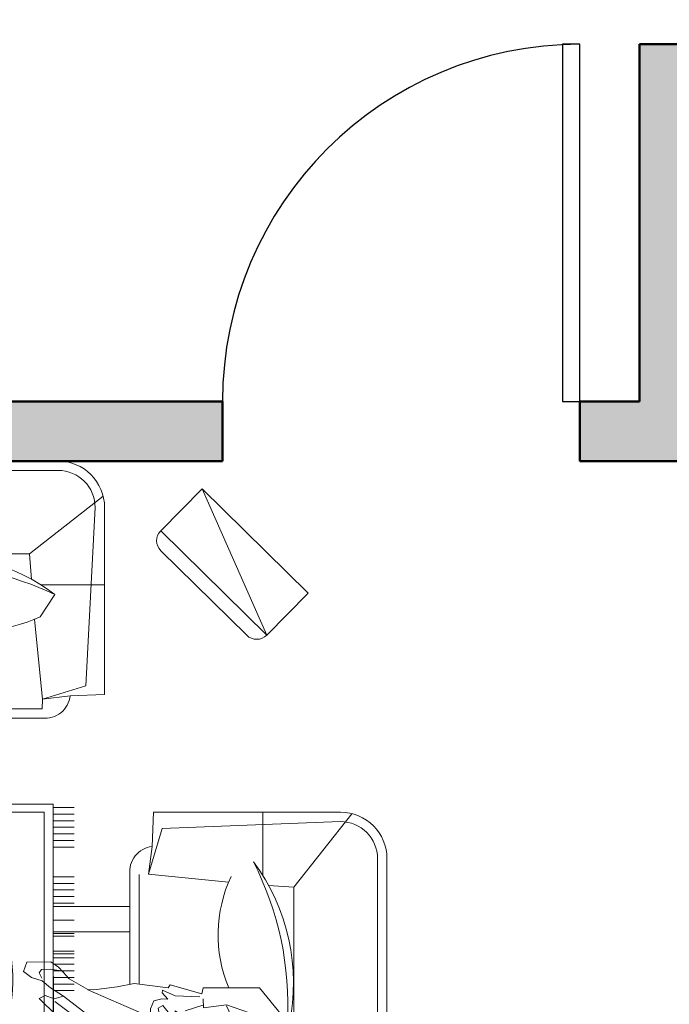
# Model space of a CAD drawing. Units: inches. Extents: x 375 to 1122, y 27 to 1069.
# Tile 70 of 155: x 601 to 667, y 400 to 499. Entities that reach past the tile are written whole.
import ezdxf

# ---------------------------------------------------------------- set-up
doc = ezdxf.new("R2010")
doc.units = ezdxf.units.IN
for name, color, linetype, lineweight in [('A-ANNO-DIMS', 2, 'Continuous', 18), ('A-WALL-PATT', 252, 'Continuous', 13), ('Doors', 150, 'Continuous', 25), ('Furniture', 30, 'Continuous', 18), ('Walls', 250, 'Continuous', 50)]:
    doc.layers.add(name, color=color, linetype=linetype, lineweight=lineweight)
doc.styles.get("Standard").update_dxf_attribs({"font": 'arial.ttf'})
doc.dimstyles.new('ISO-25', dxfattribs={"dimtxt": 12, "dimasz": 2.5, "dimexe": 1.5, "dimexo": 1.5, "dimtad": 1, "dimdec": 1, "dimlunit": 3, "dimtxsty": 'Standard', "dimblk": 'ARCHTICK', "dimcen": 2.5, "dimadec": 0, "dimazin": 0, "dimtfac": 1, "dimtdec": 1, "dimtmove": 0, "dimatfit": 3, "dimfxl": 1.5, "dimfxlon": 1, "dimarcsym": 0})

# ---------------------------------------------------------------- blocks, each defined once
blk = doc.blocks.new('*U9')
for p, q in [((-36, 0), (-36, -4)), ((0, 0), (0, -4))]:
    blk.add_line(p, q)
blk.add_lwpolyline([(0, 0), (0, 36), (-1.75, 36), (-1.75, 0)], close=True)
blk.add_arc((0, 0), 36, 90, 180)
blk = doc.blocks.new('*U11')
for p, q in [((-24, 0), (-24, -4)), ((0, 0), (0, -4))]:
    blk.add_line(p, q)
blk.add_lwpolyline([(0, 0), (0, 24), (-1.75, 24), (-1.75, 0)], close=True)
blk.add_arc((0, 0), 24, 90, 180)
blk = doc.blocks.new('A$C4DC51D13')
for p, q in [((3265.3, 2996.2), (1188.4, 2996.2)), ((1895.2, 2134), (1895.2, 2996.2)), ((2559.6, 2996.2), (2559.6, 2617.8)), ((1188.4, 2962.7), (1862.1, 2962.7)), ((1862.1, 2134), (1862.1, 2962.7)), ((1928.3, 2961.6), (2524.2, 2961.6)), ((1928.3, 2134), (1928.3, 2961.6)), ((2524.2, 2961.6), (2524.2, 2658.6)), ((2590.4, 2962.7), (2590.4, 2654.5)), ((3265.3, 2962.7), (2590.4, 2962.7)), ((277.4, 2939.6), (277.4, 2141.8)), ((943, 2103.5), (943, 2936.7)), ((1018.2, 2892.3), (232.2, 2892.3)), ((3778.5, 2897), (3631.2, 2747.3)), ((4008.9, 2375.5), (3778.5, 2897)), ((4156.2, 2525.2), (3778.5, 2897)), ((304, 2865.7), (304, 2253.3)), ((916.4, 2865.7), (304, 2865.7)), ((916.4, 2253.3), (916.4, 2865.7)), ((1290.4, 2664.8), (1028, 2870.9)), ((3163.3, 2664.8), (3425.7, 2870.9)), ((1022.9, 2163.8), (1022.9, 2830.3)), ((1056, 2830.3), (1081, 2194.8)), ((3397.7, 2830.3), (3364.5, 2194.8)), ((3430.8, 2163.8), (3430.8, 2830.3)), ((4008.9, 2375.5), (3631.2, 2747.3)), ((423.7, 2370.8), (776.6, 2723.7)), ((427.4, 2727.4), (772.8, 2367.1)), ((506.4, 2652.2), (506.4, 2704.4)), ((510.6, 2655.8), (510.6, 2706.9)), ((514.9, 2659.2), (514.9, 2709.2)), ((519.1, 2662.3), (519.1, 2711.3)), ((523.3, 2665.1), (523.3, 2713.4)), ((527.5, 2667.8), (527.5, 2715.2)), ((531.8, 2670.2), (531.8, 2717)), ((536, 2672.5), (536, 2718.7)), ((540.2, 2674.6), (540.2, 2720.2)), ((544.4, 2676.5), (544.4, 2721.6)), ((548.7, 2678.2), (548.7, 2722.9)), ((650.1, 2678.8), (650.1, 2723.3)), ((654.3, 2677.1), (654.3, 2722)), ((658.6, 2675.2), (658.6, 2720.7)), ((662.8, 2673.2), (662.8, 2719.2)), ((667, 2671), (667, 2717.6)), ((668.5, 2670.2), (668.5, 2717)), ((671.2, 2668.6), (671.2, 2715.9)), ((672.7, 2667.8), (672.7, 2715.2)), ((675.5, 2666.1), (675.5, 2714)), ((676.9, 2665.1), (676.9, 2713.4)), ((679.7, 2663.3), (679.7, 2712)), ((681.1, 2662.3), (681.1, 2711.3)), ((683.9, 2660.3), (683.9, 2709.9)), ((685.4, 2659.2), (685.4, 2709.2)), ((688.1, 2657), (688.1, 2707.7)), ((689.6, 2655.8), (689.6, 2706.9)), ((692.4, 2653.5), (692.4, 2705.3)), ((693.8, 2652.2), (693.8, 2704.4)), ((464.1, 2583.3), (464.1, 2669.7)), ((465.8, 2671.5), (534.1, 2671.5)), ((468.4, 2596.6), (468.4, 2674.3)), ((469.8, 2675.7), (542.8, 2675.7)), ((472.6, 2606.7), (472.6, 2678.5)), ((476.8, 2615), (476.8, 2682.5)), ((481, 2622.2), (481, 2686.2)), ((485.3, 2628.5), (485.3, 2689.7)), ((489.5, 2634.2), (489.5, 2693)), ((493.7, 2639.3), (493.7, 2696.1)), ((497.9, 2644), (497.9, 2699.1)), ((502.2, 2648.3), (502.2, 2701.8)), ((657.4, 2675.7), (730.4, 2675.7)), ((734.5, 2671.5), (666.1, 2671.5)), ((666.1, 2671.5), (734.5, 2671.5)), ((696.6, 2649.6), (696.6, 2702.7)), ((698, 2648.3), (698, 2701.8)), ((700.8, 2645.5), (700.8, 2700)), ((702.3, 2644), (702.3, 2699.1)), ((705, 2641), (705, 2697.2)), ((706.5, 2639.3), (706.5, 2696.1)), ((709.3, 2636), (709.3, 2694.1)), ((710.7, 2634.2), (710.7, 2693)), ((713.5, 2630.5), (713.5, 2690.9)), ((714.9, 2628.5), (714.9, 2689.7)), ((717.7, 2624.4), (717.7, 2687.4)), ((719.2, 2622.2), (719.2, 2686.2)), ((722, 2617.6), (722, 2683.8)), ((723.4, 2615), (723.4, 2682.5)), ((726.2, 2609.7), (726.2, 2679.9)), ((727.6, 2606.7), (727.6, 2678.5)), ((730.4, 2600.3), (730.4, 2675.7)), ((731.9, 2596.6), (731.9, 2674.3)), ((734.6, 2588.4), (734.6, 2671.3)), ((736.1, 2583.3), (736.1, 2669.7)), ((3631.7, 2676.6), (3938.2, 2375)), ((438.7, 2633.5), (488.9, 2633.5)), ((438.8, 2460.9), (438.8, 2633.6)), ((441, 2637.7), (492.3, 2637.7)), ((443, 2453.4), (443, 2641.1)), ((443.5, 2641.9), (496, 2641.9)), ((446.1, 2646.1), (500, 2646.1)), ((447.2, 2446.7), (447.2, 2647.8)), ((448.9, 2650.4), (504.4, 2650.4)), ((451.5, 2440.6), (451.5, 2654)), ((451.9, 2654.6), (509.2, 2654.6)), ((455.1, 2658.8), (514.4, 2658.8)), ((455.7, 2434.9), (455.7, 2659.6)), ((458.4, 2663.1), (520.2, 2663.1)), ((459.9, 2558.8), (459.9, 2664.9)), ((462, 2667.3), (526.7, 2667.3)), ((489.5, 2667.3), (489.5, 2633.5)), ((738.2, 2667.3), (673.5, 2667.3)), ((673.5, 2667.3), (738.2, 2667.3)), ((741.8, 2663.1), (680, 2663.1)), ((680, 2663.1), (741.8, 2663.1)), ((745.2, 2658.8), (685.8, 2658.8)), ((685.8, 2658.8), (745.2, 2658.8)), ((748.3, 2654.6), (691, 2654.6)), ((691, 2654.6), (748.3, 2654.6)), ((751.3, 2650.4), (695.8, 2650.4)), ((695.8, 2650.4), (751.3, 2650.4)), ((754.1, 2646.1), (700.2, 2646.1)), ((700.2, 2646.1), (754.1, 2646.1)), ((756.7, 2641.9), (704.2, 2641.9)), ((704.2, 2641.9), (756.7, 2641.9)), ((759.2, 2637.7), (707.9, 2637.7)), ((707.9, 2637.7), (759.2, 2637.7)), ((761.5, 2633.5), (711.3, 2633.5)), ((711.3, 2633.5), (761.5, 2633.5)), ((738.9, 2570.4), (738.9, 2666.6)), ((740.3, 2558.8), (740.3, 2664.9)), ((743.1, 2433.1), (743.1, 2661.5)), ((744.5, 2434.9), (744.5, 2659.6)), ((747.3, 2438.6), (747.3, 2656)), ((748.8, 2440.6), (748.8, 2654)), ((751.5, 2444.5), (751.5, 2650)), ((753, 2446.7), (753, 2647.8)), ((755.8, 2451.1), (755.8, 2643.5)), ((757.2, 2453.4), (757.2, 2641.1)), ((760, 2458.3), (760, 2636.3)), ((761.4, 2460.9), (761.4, 2633.6)), ((1283.3, 2574.2), (1290.4, 2664.8)), ((1290.4, 2664.8), (1894.7, 2664.8)), ((1798, 2530.2), (1812.1, 2637.9)), ((1895.2, 2663.7), (2557.3, 2663.7)), ((2603.6, 2664.8), (2559, 2664.8)), ((3163.3, 2664.8), (2764.7, 2664.8)), ((3170.4, 2574.2), (3163.3, 2664.8)), ((424.8, 2599.7), (469.6, 2599.7)), ((426.1, 2603.9), (471.3, 2603.9)), ((426.1, 2490.7), (426.1, 2603.9)), ((427.5, 2608.1), (473.3, 2608.1)), ((429.1, 2612.3), (475.4, 2612.3)), ((430.3, 2479), (430.3, 2615.5)), ((430.7, 2616.6), (477.7, 2616.6)), ((432.5, 2620.8), (480.2, 2620.8)), ((434.5, 2469.3), (434.5, 2625.2)), ((434.5, 2625), (482.9, 2625)), ((436.5, 2629.2), (485.8, 2629.2)), ((763.7, 2629.2), (714.4, 2629.2)), ((714.4, 2629.2), (763.7, 2629.2)), ((765.8, 2625), (717.3, 2625)), ((767.7, 2620.8), (720, 2620.8)), ((769.5, 2616.6), (722.5, 2616.6)), ((771.1, 2612.3), (724.8, 2612.3)), ((772.7, 2608.1), (726.9, 2608.1)), ((774.1, 2603.9), (728.9, 2603.9)), ((775.4, 2599.7), (730.7, 2599.7)), ((764.2, 2466.3), (764.2, 2628.2)), ((765.7, 2469.3), (765.7, 2625.2)), ((418.1, 2565.8), (460.7, 2565.8)), ((418.5, 2570.1), (461.3, 2570.1)), ((419.1, 2574.3), (462.1, 2574.3)), ((419.8, 2578.5), (462.9, 2578.5)), ((420.6, 2582.7), (464, 2582.7)), ((421.5, 2587), (465.2, 2587)), ((422.5, 2591.2), (466.5, 2591.2)), ((423.6, 2595.4), (467.9, 2595.4)), ((776.6, 2595.4), (732.3, 2595.4)), ((777.7, 2591.2), (733.7, 2591.2)), ((778.7, 2587), (735.1, 2587)), ((779.6, 2582.7), (736.2, 2582.7)), ((780.4, 2578.5), (737.3, 2578.5)), ((781.1, 2574.3), (738.2, 2574.3)), ((781.7, 2570.1), (738.9, 2570.1)), ((782.2, 2565.8), (739.6, 2565.8)), ((1895.5, 2582.2), (1932.3, 2494.6)), ((417.1, 2548.9), (459.4, 2548.9)), ((417.1, 2544.7), (459.5, 2544.7)), ((417.2, 2553.2), (459.6, 2553.2)), ((417.2, 2540.5), (459.6, 2540.5)), ((417.4, 2557.4), (459.8, 2557.4)), ((417.5, 2536.3), (459.9, 2536.3)), ((417.7, 2561.6), (460.2, 2561.6)), ((417.8, 2532), (460.3, 2532)), ((418.2, 2527.8), (460.8, 2527.8)), ((459.9, 2429.7), (459.9, 2535.7)), ((782.1, 2527.8), (739.4, 2527.8)), ((782.5, 2532), (740, 2532)), ((782.5, 2561.6), (740.1, 2561.6)), ((740.3, 2429.7), (740.3, 2535.7)), ((782.8, 2557.4), (740.4, 2557.4)), ((782.8, 2536.3), (740.4, 2536.3)), ((783, 2540.5), (740.6, 2540.5)), ((783, 2553.2), (740.7, 2553.2)), ((783.1, 2548.9), (740.8, 2548.9)), ((783.1, 2544.7), (740.8, 2544.7)), ((1022.9, 2554.4), (1249.6, 2554.4)), ((2559, 2535.8), (2557.3, 2535.8)), ((3430.8, 2554.4), (3204.1, 2554.4)), ((418.7, 2523.6), (461.4, 2523.6)), ((419.3, 2519.4), (462.2, 2519.4)), ((781, 2519.4), (738, 2519.4)), ((781.6, 2523.6), (738.8, 2523.6)), ((1200, 2520.5), (1251.9, 2440.8)), ((3253.7, 2520.5), (3201.8, 2440.8)), ((4008.9, 2375.5), (4156.2, 2525.2)), ((1243.2, 2146.7), (1272.2, 2431.8)), ((3210.5, 2146.7), (3181.5, 2431.8)), ((304, 2253.3), (916.4, 2253.3)), ((242.9, 2226.7), (1018.2, 2226.7)), ((1081, 2194.8), (1243.2, 2146.7)), ((3364.5, 2194.8), (3210.5, 2146.7)), ((1145.1, 2159.3), (1022.9, 2163.8)), ((1145.1, 2159.3), (1243.2, 2146.7)), ((1244.8, 2113), (1243.2, 2146.7)), ((2590.4, 2164.3), (2590.4, 2134)), ((3208.9, 2113), (3210.5, 2146.7)), ((3308.6, 2159.3), (3210.5, 2146.7)), ((3308.6, 2159.3), (3430.8, 2163.8)), ((498.8, 1837.1), (382.1, 2139.5)), ((1040.3, 1942.9), (421.2, 2132.6)), ((1839.5, 2113), (1244.8, 2113)), ((2308.5, 2111.9), (1950.4, 2111.9)), ((2614.2, 2113), (3208.9, 2113)), ((411.8, 2101.9), (992.6, 1890.2)), ((1839.5, 2079.9), (1244.8, 2079.9)), ((2322.1, 2078.8), (1950.4, 2078.8)), ((2614.2, 2079.9), (3208.9, 2079.9)), ((677.4, 2054.1), (612.9, 1843.6)), ((220.3, 2026), (19.3, 1370.1)), ((251.1, 2016.6), (37.1, 1314.7)), ((1009.7, 1828.1), (1040.3, 1942.9)), ((658.5, 1880), (717.8, 1809.1)), ((992.6, 1890.2), (993.4, 1733.4)), ((498.8, 1837.1), (341.4, 1323.6)), ((584.9, 1817.9), (498.8, 1837.1)), ((1009.7, 1828.1), (993.4, 1733.4)), ((1158.3, 1784.3), (1158.3, 1858.2)), ((1181.8, 1784.3), (1181.8, 1858.2)), ((1205.3, 1784.3), (1205.3, 1858.2)), ((1228.8, 1784.3), (1228.8, 1858.2)), ((1252.2, 1784.3), (1252.2, 1858.2)), ((1319.4, 1784.3), (1319.4, 1858.2)), ((1342.9, 1784.3), (1342.9, 1858.2)), ((1366.3, 1784.3), (1366.3, 1858.2)), ((1389.8, 1784.3), (1389.8, 1858.2)), ((1413.3, 1784.3), (1413.3, 1858.2)), ((1436.8, 1784.3), (1436.8, 1858.2)), ((1460.2, 1784.3), (1460.2, 1858.2)), ((1483.7, 1784.3), (1483.7, 1858.2)), ((1507.2, 1784.3), (1507.2, 1858.2)), ((1530.7, 1784.3), (1530.7, 1858.2)), ((1554.1, 1784.3), (1554.1, 1858.2)), ((1577.6, 1784.3), (1577.6, 1858.2)), ((1714.2, 1784.3), (1714.2, 1858.2)), ((1737.6, 1784.3), (1737.6, 1858.2)), ((1761.1, 1784.3), (1761.1, 1858.2)), ((1784.6, 1784.3), (1784.6, 1858.2)), ((1808.1, 1784.3), (1808.1, 1858.2)), ((1831.5, 1784.3), (1831.5, 1858.2)), ((1855, 1784.3), (1855, 1858.2)), ((1878.5, 1784.3), (1878.5, 1858.2)), ((1902, 1784.3), (1902, 1858.2)), ((2050.7, 1784.3), (2050.7, 1858.2)), ((2074.2, 1784.3), (2074.2, 1858.2)), ((2097.7, 1784.3), (2097.7, 1858.2)), ((2121.1, 1784.3), (2121.1, 1858.2)), ((2144.6, 1784.3), (2144.6, 1858.2)), ((2168.1, 1784.3), (2168.1, 1858.2)), ((2191.6, 1782.4), (2191.6, 1856.3)), ((2215, 1785.7), (2215, 1832.3)), ((2238.5, 1785.1), (2238.5, 1859)), ((2262, 1784.3), (2262, 1858.2)), ((2285.4, 1784.3), (2285.4, 1858.2)), ((2543.7, 1784.3), (2543.7, 1858.2)), ((2567.1, 1784.3), (2567.1, 1858.2)), ((2590.6, 1784.3), (2590.6, 1858.2)), ((2614.1, 1784.3), (2614.1, 1858.2)), ((2661, 1784.3), (2661, 1858.2)), ((2684.5, 1784.3), (2684.5, 1858.2)), ((2708, 1772.3), (2708, 1858.2)), ((2731.5, 1784.3), (2731.5, 1858.2)), ((2754.9, 1784.3), (2754.9, 1858.2)), ((2778.4, 1784.3), (2778.4, 1858.2)), ((2801.9, 1784.3), (2801.9, 1858.2)), ((2825.4, 1784.3), (2825.4, 1858.2)), ((2848.8, 1784.3), (2848.8, 1858.2)), ((2872.3, 1784.3), (2872.3, 1858.2)), ((2895.8, 1784.3), (2895.8, 1858.2)), ((2919.3, 1784.3), (2919.3, 1858.2)), ((2942.7, 1784.3), (2942.7, 1858.2)), ((2966.2, 1744.8), (2966.2, 1858.2)), ((2989.7, 1784.3), (2989.7, 1858.2)), ((3013.2, 1772.3), (3013.2, 1858.2)), ((3036.6, 1784.3), (3036.6, 1858.2)), ((3060.1, 1784.3), (3060.1, 1858.2)), ((3083.6, 1784.3), (3083.6, 1858.2)), ((1166.1, 1769.7), (1091.8, 1794.5)), ((1158.3, 1821.3), (1158.5, 487.7)), ((993.4, 1733.4), (720.4, 1787.6)), ((3248.4, 1772.3), (1158.5, 1772.3)), ((3248.4, 487.7), (3248.4, 1772.3)), ((3248.8, 1760.8), (3322.7, 1760.8)), ((1024.2, 1722.3), (842.3, 1125.2)), ((1024.2, 1722.3), (993.4, 1733.4)), ((1162.1, 1754.9), (1088.2, 1754.9)), ((1162.1, 1741.1), (1088.2, 1741.1)), ((1196, 511), (1196, 1744.8)), ((1196, 1744.8), (3215.6, 1744.8)), ((3215.6, 511), (3215.6, 1744.8)), ((3248.8, 1737.3), (3322.7, 1737.3)), ((3600.6, 1621.7), (3605.1, 1743.8)), ((3605.1, 1743.8), (4271.6, 1743.8)), ((3995.7, 1743.8), (3995.7, 1517.1)), ((4106.1, 1476.4), (4312.2, 1738.8)), ((873.1, 1115.8), (1055, 1712.9)), ((1162.1, 1717.6), (1088.2, 1717.6)), ((1162.1, 1708), (1088.2, 1708)), ((3248.8, 1713.8), (3322.7, 1713.8)), ((3248.8, 1690.4), (3322.7, 1690.4)), ((3636.1, 1685.8), (3588, 1523.6)), ((4271.6, 1710.7), (3636.1, 1685.8)), ((1162.1, 1684.5), (1088.2, 1684.5)), ((3248.8, 1666.9), (3322.7, 1666.9)), ((3248.8, 1643.4), (3322.7, 1643.4)), ((3248.8, 1619.9), (3322.7, 1619.9)), ((3600.6, 1621.7), (3588, 1523.6)), ((4404, 1578.3), (4404, 904.6)), ((4437.5, 165.9), (4437.5, 1578.3)), ((1701.7, 1530), (1701.7, 911.2)), ((3248.8, 1513.8), (3322.7, 1513.8)), ((3248.8, 1513.3), (3322.7, 1513.3)), ((3521.2, 1130.7), (3521.2, 1521.9)), ((3554.3, 1131.4), (3554.3, 1521.9)), ((3588, 1523.6), (3873.1, 1494.5)), ((1162.1, 1492.9), (1088.2, 1492.9)), ((1162.1, 1483.3), (1088.2, 1483.3)), ((1737.7, 1483.1), (1737.7, 911.2)), ((2593.1, 907.9), (2593.1, 1490.3)), ((2629.1, 907.9), (2629.1, 1503.1)), ((3248.8, 1490.4), (3322.7, 1490.4)), ((3248.8, 1489.9), (3322.7, 1489.9)), ((4015.5, 1483.4), (4106.1, 1476.4)), ((4106.1, 1476.4), (4106.1, 872.1)), ((1162.1, 1459.8), (1088.2, 1459.8)), ((1162.1, 1446), (1088.2, 1446)), ((2674.6, 1449.9), (1641, 1449.9)), ((1888.1, 1449.9), (1701.7, 1263.5)), ((1856.2, 1449.9), (1701.7, 1295.4)), ((1715.1, 1449.9), (1701.7, 1436.5)), ((2343.3, 1449.9), (1855.3, 961.9)), ((2629.1, 1449), (2142, 961.9)), ((2325.1, 1449.9), (2154.2, 1279.1)), ((2461.6, 1449.9), (2177, 1165.3)), ((3248.8, 1466.9), (3322.7, 1466.9)), ((3248.8, 1443.4), (3322.7, 1443.4)), ((1162.1, 1412.8), (1088.2, 1412.8)), ((2674.6, 1413.9), (1641, 1413.9)), ((3248.8, 1419.9), (3322.7, 1419.9)), ((3250, 1407.8), (3519, 1407.8)), ((6.3, 1324.2), (19.3, 1370.2)), ((1162.1, 1399), (1088.2, 1399)), ((1162.1, 1375.5), (1088.2, 1375.5)), ((479.3, 1327.3), (375.2, 1344.9)), ((1162.1, 1352.1), (1088.2, 1352.1)), ((1162.1, 1342.9), (1088.2, 1342.9)), ((1162.1, 1342.4), (1088.2, 1342.4)), ((3248.8, 1359), (3322.7, 1359)), ((342.8, 1324.6), (76.7, 1139.6)), ((843, 1127.6), (342.8, 1324.6)), ((1162.1, 1319.4), (1088.2, 1319.4)), ((1162.1, 1318.9), (1088.2, 1318.9)), ((3248.8, 990.8), (3248.4, 1328.4)), ((3248.8, 1312.1), (3322.7, 1312.1)), ((3248.8, 1302.3), (3322.7, 1302.3)), ((3250, 1317.8), (3519, 1317.8)), ((369.2, 1044.8), (442.9, 1285.2)), ((1162.1, 1296), (1088.2, 1296)), ((1162.1, 1295.5), (1088.2, 1295.5)), ((1196, 1272.5), (1088.2, 1272.5)), ((1162.1, 1272), (1088.2, 1272)), ((2629.1, 1280.5), (2310.5, 961.9)), ((1162.1, 1249), (1088.2, 1249)), ((1162.1, 1248.5), (1088.2, 1248.5)), ((3248.8, 1249), (3322.7, 1249)), ((3248.8, 1248.5), (3322.7, 1248.5)), ((3248.8, 1239.3), (3322.7, 1239.3)), ((3248.8, 1238.8), (3322.7, 1238.8)), ((1162.1, 1225.5), (1088.2, 1225.5)), ((1162.1, 1202.1), (1088.2, 1202.1)), ((3248.8, 1225.5), (3322.7, 1225.5)), ((3248.8, 1202.1), (3322.7, 1202.1)), ((1196, 1178.6), (1088.2, 1178.6)), ((3248.8, 1178.6), (3322.7, 1178.6)), ((122.4, 1154.1), (719.7, 996.3)), ((719.7, 996.3), (810.6, 1133.2)), ((771, 1045.7), (810.6, 1133.2)), ((842.3, 1125.2), (810.6, 1133.2)), ((1162.1, 1155.1), (1088.2, 1155.1)), ((1162.1, 1131.6), (1088.2, 1131.6)), ((1728.6, 1158.4), (1701.7, 1131.5)), ((3248.8, 1155.1), (3322.7, 1155.1)), ((3248.8, 1131.6), (3322.7, 1131.6)), ((732, 933.5), (112.9, 1123.3)), ((1162.1, 1108.2), (1088.2, 1108.2)), ((3248.8, 1108.2), (3322.7, 1108.2)), ((1162.1, 1084.7), (1088.2, 1084.7)), ((1196, 1061.2), (1088.2, 1061.2)), ((771, 1045.7), (732, 933.5)), ((1162.1, 1037.7), (1088.2, 1037.7)), ((1648.3, 1019.6), (2616.7, 1019.6)), ((1926.6, 1051.5), (1837.1, 961.9)), ((1162.1, 1014.3), (1088.2, 1014.3)), ((2006.3, 994.6), (1973.6, 961.9)), ((2629.1, 1012), (2579, 961.9)), ((3248.8, 1014.3), (3322.7, 1014.3)), ((3248.8, 990.8), (3322.7, 990.8)), ((1196, 967.3), (1088.2, 967.3)), ((1648.3, 961.9), (2681.9, 961.9)), ((2459.2, 974.1), (2447, 961.9)), ((3248.8, 967.3), (3322.7, 967.3)), ((1162.1, 943.8), (1088.2, 943.8)), ((1162.1, 920.4), (1088.2, 920.4)), ((3248.8, 943.8), (3322.7, 943.8)), ((3248.8, 920.4), (3322.7, 920.4)), ((4097.4, 904.6), (4404, 904.6)), ((1196, 860.5), (1088.2, 860.5)), ((4106.1, 871.5), (4437.5, 871.5)), ((1162.1, 837), (1088.2, 837)), ((1162.1, 813.5), (1088.2, 813.5)), ((3521.2, 816.9), (3521.2, 222.3)), ((3554.3, 816.9), (3554.3, 222.3)), ((4404, 840.7), (4110.5, 840.7)), ((4404, 165.9), (4404, 840.7)), ((1162.1, 790), (1031.8, 790)), ((1196, 766.6), (1088.2, 766.6)), ((1162.1, 743.1), (1088.2, 743.1)), ((1162.1, 719.6), (1088.2, 719.6)), ((4106.1, 267.8), (4106.1, 666.5)), ((1162.1, 627.8), (1088.2, 627.8)), ((1162.1, 604.4), (1088.2, 604.4)), ((3248.8, 627.8), (3322.7, 627.8)), ((3248.8, 604.4), (3322.7, 604.4)), ((1162.1, 580.9), (1034.2, 580.9)), ((3248.8, 580.9), (3322.7, 580.9)), ((1162.1, 557.4), (1088.2, 557.4)), ((1162.1, 533.9), (1088.2, 533.9)), ((3248.8, 557.4), (3322.7, 557.4)), ((3248.8, 533.9), (3322.7, 533.9)), ((1162.1, 510.5), (1088.2, 510.5)), ((1162, 495.1), (1116.6, 429)), ((3215.6, 511), (1196, 511)), ((1334.6, 511), (1334.6, 402.4)), ((1381.6, 511), (1381.6, 402.4)), ((2059.5, 511), (2059.5, 402.4)), ((2106.4, 511), (2106.4, 402.4)), ((2669.8, 511), (2669.8, 402.4)), ((3244.9, 495.1), (3290.3, 429)), ((3248.8, 510.5), (3322.7, 510.5)), ((1158.5, 487.7), (3248.4, 487.7)), ((1167.1, 476.3), (1167.1, 402.4)), ((1190.6, 476.3), (1190.6, 402.4)), ((1214, 476.3), (1214, 402.4)), ((1237.5, 476.3), (1237.5, 402.4)), ((1311.1, 487.7), (1311.1, 402.4)), ((1358.1, 476.3), (1358.1, 402.4)), ((1405, 476.3), (1405, 402.4)), ((1428.5, 487.7), (1428.5, 402.4)), ((1452, 476.3), (1452, 402.4)), ((1475.5, 476.3), (1475.5, 402.4)), ((1498.9, 487.7), (1498.9, 402.4)), ((1522.4, 487.7), (1522.4, 402.4)), ((1545.9, 476.3), (1545.9, 402.4)), ((1569.4, 476.3), (1569.4, 402.4)), ((1592.8, 476.3), (1592.8, 402.4)), ((1616.3, 476.3), (1616.3, 402.4)), ((1639.8, 476.3), (1639.8, 402.4)), ((1663.3, 487.7), (1663.3, 402.4)), ((1757.8, 487.7), (1757.8, 402.4)), ((1781.3, 487.7), (1781.3, 402.4)), ((1804.8, 476.3), (1804.8, 402.4)), ((1828.2, 476.3), (1828.2, 402.4)), ((1851.7, 476.3), (1851.7, 402.4)), ((1875.2, 476.3), (1875.2, 402.4)), ((1898.7, 476.3), (1898.7, 402.4)), ((1922.1, 487.7), (1922.1, 402.4)), ((2036, 487.7), (2036, 402.4)), ((2082.9, 476.3), (2082.9, 402.4)), ((2129.9, 476.3), (2129.9, 402.4)), ((2153.4, 487.7), (2153.4, 402.4)), ((2176.8, 476.3), (2176.8, 402.4)), ((2200.3, 476.3), (2200.3, 402.4)), ((2223.8, 487.7), (2223.8, 402.4)), ((2247.2, 487.7), (2247.2, 402.4)), ((2270.7, 476.3), (2270.7, 402.4)), ((2294.2, 476.3), (2294.2, 402.4)), ((2317.7, 476.3), (2317.7, 402.4)), ((2341.1, 476.3), (2341.1, 402.4)), ((2364.6, 476.3), (2364.6, 402.4)), ((2388.1, 487.7), (2388.1, 402.4)), ((2411.6, 476.3), (2411.6, 402.4)), ((2435, 476.3), (2435, 402.4)), ((2458.5, 476.3), (2458.5, 402.4)), ((2482, 487.7), (2482, 402.4)), ((2505.5, 487.7), (2505.5, 402.4)), ((2528.9, 476.3), (2528.9, 402.4)), ((2552.4, 476.3), (2552.4, 402.4)), ((2575.9, 476.3), (2575.9, 402.4)), ((2599.4, 476.3), (2599.4, 402.4)), ((2622.8, 476.3), (2622.8, 402.4)), ((2646.3, 476.3), (2646.3, 402.4)), ((2693.3, 476.3), (2693.3, 402.4)), ((2716.7, 476.3), (2716.7, 402.4)), ((2738, 476.3), (2738, 402.4)), ((2740.2, 487.7), (2740.2, 402.4)), ((2761.5, 476.3), (2761.5, 402.4)), ((2763.7, 476.3), (2763.7, 402.4)), ((2784.9, 487.7), (2784.9, 402.4)), ((2787.2, 476.3), (2787.2, 402.4)), ((2808.4, 476.3), (2808.4, 402.4)), ((2810.6, 476.3), (2810.6, 402.4)), ((2831.9, 476.3), (2831.9, 402.4)), ((2834.1, 476.3), (2834.1, 402.4)), ((2855.4, 476.3), (2855.4, 402.4)), ((2857.6, 476.3), (2857.6, 402.4)), ((2878.8, 476.3), (2878.8, 402.4)), ((2881.1, 476.3), (2881.1, 402.4)), ((2902.3, 476.3), (2902.3, 402.4)), ((2904.5, 487.7), (2904.5, 402.4)), ((2925.8, 476.3), (2925.8, 402.4)), ((2928, 476.3), (2928, 402.4)), ((2949.3, 476.3), (2949.3, 402.4)), ((2951.5, 476.3), (2951.5, 402.4)), ((2972.7, 476.3), (2972.7, 402.4)), ((2975, 476.3), (2975, 402.4)), ((2996.2, 476.3), (2996.2, 402.4)), ((2998.4, 476.3), (2998.4, 402.4)), ((3019.7, 476.3), (3019.7, 402.4)), ((3021.9, 487.7), (3021.9, 402.4)), ((3043.2, 476.3), (3043.2, 402.4)), ((3045.4, 476.3), (3045.4, 402.4)), ((3066.6, 476.3), (3066.6, 402.4)), ((3068.9, 476.3), (3068.9, 402.4)), ((3092.3, 476.3), (3092.3, 402.4)), ((3092.7, 484.5), (3092.7, 410.6)), ((3115.8, 476.3), (3115.8, 402.4)), ((3116.2, 484.5), (3116.2, 410.6)), ((3202.2, 476.3), (3202.2, 402.4)), ((3225.7, 476.3), (3225.7, 402.4)), ((3249.2, 476.3), (3249.2, 402.4)), ((3588, 220.6), (3873.1, 249.7)), ((4015.5, 260.8), (4106.1, 267.8)), ((4106.1, 267.8), (4312.2, 5.4)), ((3636.1, 66.6), (3588, 220.6)), ((3961.8, 177.4), (3882.1, 229.3)), ((3995.7, 0.4), (3995.7, 227)), ((3600.6, 122.5), (3605.1, 0.4)), ((4271.6, 33.5), (3636.1, 66.6)), ((3605.1, 0.4), (4271.6, 0.4))]:
    blk.add_line(p, q)
at = {"linetype": 'ByBlock'}
for points in [[(2342.9, 1843.9), (2352.5, 1810.4), (2340.1, 1777.7), (2351.8, 1757), (2412.3, 1818), (2433.1, 1866.4), (2453.1, 1889.5), (2436, 1914.7), (2407.6, 1926.2), (2433.7, 1959.9), (2473.1, 2048.3), (2530.6, 2101.1), (2625.9, 2180.3), (2669, 2174.2), (2748.1, 2315.4), (2745.8, 2342.6), (2801.2, 2404.9), (2823.9, 2479.6), (2818.4, 2529.9), (2775.1, 2571.7), (2782.4, 2583.3), (2765.2, 2658.8), (2714.5, 2706.9), (2634.6, 2708.6), (2571.9, 2652.6), (2548.8, 2649.4), (2474, 2672.1), (2312.9, 2542.1), (2312.9, 2341.6), (2333.9, 2336.4), (2302, 2223.9), (2313.6, 2216.6), (2297.4, 2095.7), (2309.3, 2034.9), (2320.2, 1952), (2319.3, 1929.9), (2280.8, 1863.6), (2257.7, 1842.4), (2239.2, 1825.7), (2220.1, 1798.2), (2221.6, 1713.1), (2254.3, 1700.7), (2275.9, 1729.8), (2288.6, 1768), (2313.7, 1797.6)], [(3285.2, 1088.3), (3251.7, 1078.6), (3219, 1091.1), (3198.3, 1079.4), (3259.3, 1018.8), (3307.7, 998), (3330.8, 978), (3356, 995.1), (3367.5, 1023.6), (3401.2, 997.5), (3489.6, 958), (3542.4, 900.5), (3621.6, 805.3), (3615.5, 762.2), (3756.7, 683), (3783.9, 685.3), (3846.2, 629.9), (3920.9, 607.2), (3971.2, 612.7), (4013, 656), (4024.6, 648.7), (4100.1, 665.9), (4148.2, 716.6), (4149.9, 796.5), (4093.9, 859.3), (4090.7, 882.4), (4113.4, 957.1), (3983.4, 1118.2), (3782.9, 1118.2), (3777.7, 1097.2), (3665.2, 1129.2), (3657.9, 1117.6), (3537, 1133.7), (3476.2, 1121.9), (3393.3, 1110.9), (3371.2, 1111.9), (3304.9, 1150.4), (3283.7, 1173.4), (3267, 1191.9), (3239.5, 1211), (3154.4, 1209.5), (3142, 1176.8), (3171.1, 1155.3), (3209.3, 1142.5), (3238.9, 1117.5)]]:
    blk.add_lwpolyline(points, close=True, dxfattribs=at)
for points in [[(2563.4, 2654.7), (2512.2, 2609.3), (2506.2, 2548.3), (2540.1, 2504.4), (2576.9, 2490.9), (2579.8, 2539.3), (2598.7, 2543.6), (2636.7, 2516.4), (2690.3, 2516.7), (2731.2, 2520.1), (2758.5, 2540.1), (2773, 2563.3)], [(2629.1, 2357.8), (2507, 2405.5), (2433.2, 2450.3), (2445.5, 2500.8), (2478.9, 2546.1), (2402.4, 2506.9), (2373.4, 2424.8), (2384.4, 2341.9), (2352.8, 2340.7)], [(2712.3, 2515.8), (2652.7, 2472.4), (2603.2, 2489), (2580, 2503.6)], [(2738, 2438.2), (2699.2, 2425.4), (2742.4, 2401.4), (2680.4, 2403.2), (2604.1, 2328.3), (2519.2, 2273.3), (2529.8, 2261.8), (2402.7, 2252.7), (2395.4, 2241.1), (2431.1, 2241.3), (2375.7, 2196.9), (2385.2, 2181.2), (2474.4, 2199.5), (2549.9, 2234.6), (2596.2, 2223.2), (2730.1, 2333.1)], [(2433.2, 2450.3), (2377.6, 2423.8)], [(2409.5, 2153), (2387.5, 2153.9), (2359, 2165.4), (2352.6, 2193.7), (2353.5, 2215.7), (2330.5, 2194.6), (2322.1, 2196.7), (2341.8, 2240.9), (2345.5, 2329.1)], [(2374.9, 2339.8), (2395.2, 2276.9)], [(2613.2, 2183.4), (2541.6, 2218.8)], [(2431.4, 2187.8), (2379.5, 2066.7), (2320.2, 1929.7)], [(2407.6, 1926.2), (2342.9, 1843.9)], [(2412.9, 1911.5), (2401.6, 1865.2), (2361.9, 1812.5)], [(2279.2, 1765.9), (2259.2, 1757.4), (2247.6, 1764.7), (2246.4, 1796.2), (2253.5, 1843.5)], [(3207.2, 1152), (3198.7, 1171.9), (3206, 1183.5), (3237.5, 1184.7), (3284.8, 1177.6)], [(3367.5, 1023.6), (3285.2, 1088.3)], [(3629.1, 999.7), (3508, 1051.6), (3371, 1110.9)], [(3594.3, 1021.6), (3595.2, 1043.7), (3606.7, 1072.1), (3635, 1078.6), (3657, 1077.6), (3635.9, 1100.6), (3638, 1109.1), (3682.2, 1089.3), (3770.4, 1085.6)], [(3352.8, 1018.2), (3306.5, 1029.5), (3253.8, 1069.2)], [(3879.5, 693.2), (3866.7, 732), (3842.7, 688.8), (3844.5, 750.8), (3769.6, 827.1), (3714.6, 911.9), (3703.1, 901.3), (3694, 1028.4), (3682.4, 1035.7), (3682.6, 1000), (3638.2, 1055.5), (3622.5, 1045.9), (3640.8, 956.7), (3675.9, 881.2), (3664.5, 834.9), (3774.4, 701)], [(3781.1, 1056.2), (3718.2, 1035.9)], [(3799.1, 802), (3846.8, 924.2), (3891.6, 998), (3942.1, 985.6), (3987.4, 952.2), (3948.2, 1028.7), (3866.1, 1057.7), (3783.2, 1046.8), (3782, 1078.3)], [(3891.6, 998), (3865.1, 1053.5)], [(4096, 867.7), (4050.6, 918.9), (3989.6, 924.9), (3945.7, 891.1), (3932.2, 854.2), (3980.6, 851.3), (3984.9, 832.4), (3957.7, 794.4), (3958, 740.9), (3961.4, 699.9), (3981.4, 672.7), (4004.6, 658.1)], [(3624.7, 817.9), (3660.1, 889.6)], [(3957.1, 718.8), (3913.7, 778.5), (3930.3, 827.9), (3944.9, 851.1)]]:
    blk.add_lwpolyline(points, dxfattribs=at)
for centre, radius in [((600.1, 2547.3), 183), ((600.1, 2547.3), 140.7), ((1803.2, 1372.6), 25.7), ((2527.6, 1372.6), 25.7), ((1803.2, 1039.3), 25.7), ((2527.6, 1039.3), 25.7), ((2817.9, 923.4), 31.7), ((2095.7, 858), 41)]:
    blk.add_circle(centre, radius)
for centre, radius, start, end in [((1188.4, 2830.3), 165.9, 90, 180), ((3265.3, 2830.3), 165.9, 0, 90), ((1188.4, 2830.3), 132.4, 90, 180), ((3265.3, 2830.3), 132.4, 0, 90), ((3666.8, 2712.2), 50, 135.4503, 225.4503), ((1626.8, 1949.8), 712.7, 74.928, 126.7929), ((1707.9, 1527), 1115.8, 84.6406, 117.0804), ((2210.2, 1780.8), 852.5, 76.866, 111.6839), ((2192.2, 2032.6), 624.6, 69.4145, 118.3621), ((2633.9, 373.6), 2292.5, 91.8726, 91.9144), ((2832.8, 1963.1), 698.5, 52.9389, 95.0789), ((2713.3, 1357.7), 1282.3, 65.0725, 87.2152), ((1459.9, 2882.7), 488.4, 244.7866, 313.8058), ((2216, 2892.1), 488.4, 234.4888, 282.1285), ((2993.8, 2882.7), 488.4, 248.2152, 295.2134), ((3973.2, 2410.6), 50, 225.4503, 315.4503), ((1234.5, 2169.3), 90, 186.4251, 276.5821), ((3219.2, 2169.3), 90, 263.4179, 353.5749), ((374.1, 1978.9), 160.8, 72.9571, 162.9571), ((374.1, 1978.9), 128.6, 72.9571, 162.9571), ((1839.5, 2135.1), 22.1, 270, 0), ((1839.5, 2135.1), 55.2, 270, 0), ((1950.4, 2134), 55.2, 180, 270), ((1950.4, 2134), 22.1, 180, 270), ((2619.6, 2148.3), 68.5, 191.0595, 265.4426), ((2614.2, 2135.1), 22.1, 180, 270), ((1584.7, 1047), 1245.7, 138.0296, 166.1636), ((1067.1, 1321), 692.3, 126.1642, 178.0291), ((974.8, 1747.9), 87.4, 336.375, 66.532), ((248.2, 1741.7), 474.4, 299.1514, 8.1705), ((4271.6, 1578.3), 165.9, 0, 90), ((4271.6, 1578.3), 132.4, 0, 90), ((944.2, 1233.8), 467.1, 309.4804, 56.621), ((3610.6, 1532.2), 90, 96.4251, 186.5821), ((3383, 1136.2), 721.4, 348.1046, 36.6442), ((2968.3, 1058.8), 1115.8, 356.7543, 27.0804), ((4324, 1306.8), 488.4, 154.7866, 202.7137), ((160.1, 1277), 160.8, 162.9571, 252.9571), ((160.1, 1277), 128.6, 162.9571, 252.9571), ((2517.5, 1143.6), 586.7, 287.3395, 13.1463), ((787.1, 1131.7), 87.4, 259.3822, 349.5393), ((2356.9, 1798.1), 1287.8, 212.1153, 261.9323), ((-29968.2, -49615.7), 59944, 56.743614, 57.623407), ((3404.4, 598.4), 698.5, 322.9389, 5.0789), ((2799, 717.9), 1282.3, 335.0725, 357.2152), ((4324, 437.4), 488.4, 158.2152, 205.2134), ((2591.9, -2109.1), 2694.5, 80.9842, 100.0261), ((3610.6, 212), 90, 173.4179, 263.5749), ((4271.6, 165.9), 132.4, 270, 0), ((4271.6, 165.9), 165.9, 270, 0)]:
    blk.add_arc(centre, radius, start, end)
blk = doc.blocks.new('_ArchTick')
at = {"color": 0, "linetype": 'ByBlock', "const_width": 0.15}
blk.add_lwpolyline([(-0.5, -0.5), (0.5, 0.5)], dxfattribs=at)
blk = doc.blocks.new('*D44')
at = {"layer": 'A-ANNO-DIMS', "color": 0, "lineweight": -2, "transparency": 16777216}
for p, q in [((541.855, 504.434), (541.855, 501.434)), ((607.16, 504.434), (607.16, 501.434)), ((541.855, 502.934), (607.16, 502.934)), ((607.16, 502.934), (712.018, 502.934))]:
    blk.add_line(p, q, dxfattribs=at)
at = {"layer": 'Defpoints', "color": 0, "transparency": 16777216}
for p in [(541.855, 513.055), (607.16, 513.055), (607.16, 502.934)]:
    blk.add_point(p, dxfattribs=at)
at = {"layer": 'A-ANNO-DIMS', "color": 0, "lineweight": -2, "transparency": 16777216, "xscale": 2.5, "yscale": 2.5, "zscale": 2.5, "rotation": 180}
blk.add_blockref('_ArchTick', (541.855, 502.934), dxfattribs=at)
at = {"layer": 'A-ANNO-DIMS', "color": 0, "lineweight": -2, "transparency": 16777216, "xscale": 2.5, "yscale": 2.5, "zscale": 2.5}
blk.add_blockref('_ArchTick', (607.16, 502.934), dxfattribs=at)
at = {"layer": 'A-ANNO-DIMS', "color": 0, "transparency": 16777216, "insert": (660.839, 509.764), "char_height": 12, "attachment_point": 5}
blk.add_mtext('5\'-5 1/2" TYP.', dxfattribs=at)
blk = doc.blocks.new('*D82')
at = {"layer": 'A-ANNO-DIMS', "color": 0, "lineweight": -2, "transparency": 16777216}
for p, q in [((401.507, 1009.528), (398.507, 1009.528)), ((400.007, 160.528), (400.007, 1009.528)), ((401.507, 160.528), (398.507, 160.528))]:
    blk.add_line(p, q, dxfattribs=at)
at = {"layer": 'Defpoints', "color": 0, "transparency": 16777216}
for p in [(400.007, 1009.528), (630.534, 1009.528), (630.534, 160.528)]:
    blk.add_point(p, dxfattribs=at)
at = {"layer": 'A-ANNO-DIMS', "color": 0, "lineweight": -2, "transparency": 16777216, "xscale": 2.5, "yscale": 2.5, "zscale": 2.5}
for p, rotation in [((400.007, 1009.528), 90), ((400.007, 160.528), 270)]:
    blk.add_blockref('_ArchTick', p, dxfattribs=dict(at, rotation=rotation))
at = {"layer": 'A-ANNO-DIMS', "color": 0, "transparency": 16777216, "insert": (393.255, 585.028), "char_height": 12, "attachment_point": 5, "rotation": 90}
blk.add_mtext('70\'-9"', dxfattribs=at)
blk = doc.blocks.new('*D92')
at = {"layer": 'A-ANNO-DIMS', "color": 0, "lineweight": -2, "transparency": 16777216}
for p, q in [((621.507, 1052.528), (621.507, 1055.528)), ((657.507, 1052.528), (657.507, 1055.528)), ((621.507, 1054.028), (657.507, 1054.028))]:
    blk.add_line(p, q, dxfattribs=at)
at = {"layer": 'Defpoints', "color": 0, "transparency": 16777216}
for p in [(657.507, 1054.028), (621.507, 460.528), (657.507, 460.528)]:
    blk.add_point(p, dxfattribs=at)
at = {"layer": 'A-ANNO-DIMS', "color": 0, "lineweight": -2, "transparency": 16777216, "xscale": 2.5, "yscale": 2.5, "zscale": 2.5, "rotation": 180}
blk.add_blockref('_ArchTick', (621.507, 1054.028), dxfattribs=at)
at = {"layer": 'A-ANNO-DIMS', "color": 0, "lineweight": -2, "transparency": 16777216, "xscale": 2.5, "yscale": 2.5, "zscale": 2.5}
blk.add_blockref('_ArchTick', (657.507, 1054.028), dxfattribs=at)
at = {"layer": 'A-ANNO-DIMS', "color": 0, "transparency": 16777216, "insert": (639.507, 1060.784), "char_height": 12, "attachment_point": 5}
blk.add_mtext('3\'-0"', dxfattribs=at)

msp = doc.modelspace()

# ---------------------------------------------------------------- hatches: boundary and pattern name
at = {"layer": 'A-WALL-PATT'}
h = msp.add_hatch(color=256, dxfattribs=at)
h.dxf.hatch_style = 1
h.paths.add_polyline_path([(962.007, 388.528), (989.007, 388.528), (989.007, 394.528), (962.007, 394.528), (932.007, 394.528), (932.007, 397.528), (923.007, 397.528), (923.007, 394.528), (842.007, 394.528), (842.007, 334.528), (839.507, 334.528), (839.507, 328.528), (854.007, 328.528), (854.007, 334.528), (848.007, 334.528), (848.007, 388.528), (953.007, 388.528), (953.007, 356.081), (962.007, 356.081), (962.007, 358.554), (989.007, 358.554), (989.007, 364.554), (962.007, 364.554)])
h.paths.add_polyline_path([(989.007, 502.528), (932.007, 502.528), (932.007, 583.528), (932.007, 593.528), (923.007, 593.528), (923.007, 583.528), (854.007, 583.528), (854.007, 556.528), (863.007, 556.528), (863.007, 574.528), (923.007, 574.528), (923.007, 502.528), (863.007, 502.528), (863.007, 520.528), (854.007, 520.528), (854.007, 502.528), (773.007, 502.528), (773.007, 493.528), (788.007, 493.528), (788.007, 402.028), (722.007, 402.028), (722.007, 373.528), (728.007, 373.528), (728.007, 396.028), (788.007, 396.028), (788.007, 373.528), (794.007, 373.528), (794.007, 430.528), (814.007, 430.528), (814.007, 436.528), (794.007, 436.528), (794.007, 493.528), (923.007, 493.528), (923.007, 487.528), (932.007, 487.528), (932.007, 493.528), (983.007, 493.528), (983.007, 473.528), (989.007, 473.528)])
h.paths.add_polyline_path([(797.007, 325.528), (805.007, 325.528), (805.007, 328.528), (807.507, 328.528), (807.507, 334.528), (791.007, 334.528), (791.007, 226.528), (770.757, 226.528), (770.757, 217.528), (791.007, 217.528), (791.007, 187.528), (855.007, 187.528), (855.007, 196.528), (797.007, 196.528)])
h.paths.add_polyline_path([(989.007, 238.528), (962.007, 238.528), (962.007, 256.424), (953.007, 256.424), (953.007, 229.528), (980.007, 229.528), (980.007, 196.528), (915.007, 196.528), (915.007, 187.528), (989.007, 187.528)])
h.paths.add_polyline_path([(962.007, 334.528), (884.007, 334.528), (884.007, 328.528), (918.007, 328.528), (918.007, 325.528), (932.007, 325.528), (932.007, 328.528), (953.007, 328.528), (953.007, 304.424), (962.007, 304.424)])
h.paths.add_polyline_path([(606.507, 283.528), (609.507, 283.528), (609.507, 289.528), (600.507, 289.528), (600.507, 196.528), (578.507, 196.528), (578.507, 187.528), (606.507, 187.528), (606.507, 196.528)])
h.paths.add_polyline_path([(666.507, 292.528), (660.507, 292.528), (660.507, 289.528), (633.507, 289.528), (633.507, 283.528), (660.507, 283.528), (660.507, 196.528), (628.007, 196.528), (628.007, 187.528), (630.534, 187.528), (630.534, 160.528), (636.534, 160.528), (636.534, 187.528), (660.507, 187.528), (660.507, 160.528), (666.507, 160.528), (666.507, 217.528), (686.757, 217.528), (686.757, 226.528), (666.507, 226.528)])
h.paths.add_polyline_path([(480.507, 256.424), (471.507, 256.424), (471.507, 238.528), (444.507, 238.528), (444.507, 187.528), (518.507, 187.528), (518.507, 196.528), (453.507, 196.528), (453.507, 229.528), (480.507, 229.528)])
h.paths.add_polyline_path([(480.507, 328.528), (652.507, 328.528), (652.507, 325.528), (660.507, 325.528), (660.507, 322.528), (666.507, 322.528), (666.507, 334.528), (507.507, 334.528), (507.507, 360.528), (498.507, 360.528), (498.507, 334.528), (471.507, 334.528), (471.507, 304.424), (480.507, 304.424)])
h.paths.add_polyline_path([(507.507, 484.528), (498.507, 484.528), (498.507, 444.528), (507.507, 444.528), (507.507, 454.528), (621.507, 454.528), (621.507, 460.528), (507.507, 460.528)])
h.paths.add_polyline_path([(672.507, 604.528), (683.257, 604.528), (683.257, 613.528), (669.507, 613.528), (669.507, 649.528), (663.507, 649.528), (663.507, 589.528), (507.507, 589.528), (507.507, 613.528), (498.507, 613.528), (498.507, 556.528), (507.507, 556.528), (507.507, 580.528), (663.507, 580.528), (663.507, 520.528), (669.507, 520.528), (669.507, 556.528), (683.257, 556.528), (683.257, 565.528), (672.507, 565.528)])
h.paths.add_polyline_path([(731.007, 667.528), (734.007, 667.528), (734.007, 676.528), (728.007, 676.528), (728.007, 715.528), (657.507, 715.528), (657.507, 709.528), (663.507, 709.528), (663.507, 673.528), (669.507, 673.528), (669.507, 709.528), (722.007, 709.528), (722.007, 613.528), (704.757, 613.528), (704.757, 604.528), (722.007, 604.528), (722.007, 565.528), (704.757, 565.528), (704.757, 556.528), (722.007, 556.528), (722.007, 502.528), (722.007, 460.528), (669.507, 460.528), (669.507, 496.528), (663.507, 496.528), (663.507, 460.528), (657.507, 460.528), (657.507, 454.528), (728.007, 454.528), (728.007, 493.528), (734.007, 493.528), (734.007, 502.528), (731.007, 502.528)])
h.paths.add_polyline_path([(986.007, 718.528), (959.007, 718.528), (959.007, 727.528), (950.007, 727.528), (950.007, 709.528), (977.007, 709.528), (977.007, 676.528), (794.007, 676.528), (794.007, 805.528), (802.007, 805.528), (802.007, 808.528), (804.507, 808.528), (804.507, 814.528), (788.007, 814.528), (788.007, 774.028), (728.007, 774.028), (728.007, 796.528), (722.007, 796.528), (722.007, 768.028), (788.007, 768.028), (788.007, 676.528), (773.007, 676.528), (773.007, 667.528), (923.007, 667.528), (923.007, 657.528), (932.007, 657.528), (932.007, 667.528), (986.007, 667.528)])
h.paths.add_polyline_path([(621.507, 715.528), (507.507, 715.528), (507.507, 733.528), (498.507, 733.528), (498.507, 715.528), (498.507, 685.528), (507.507, 685.528), (507.507, 709.528), (621.507, 709.528)])
h.paths.add_polyline_path([(666.507, 847.028), (660.507, 847.028), (660.507, 844.528), (652.507, 844.528), (652.507, 841.528), (480.507, 841.528), (480.507, 859.528), (471.507, 859.528), (471.507, 835.528), (498.507, 835.528), (498.507, 817.528), (507.507, 817.528), (507.507, 835.528), (666.507, 835.528)])
h.paths.add_polyline_path([(480.507, 940.528), (453.507, 940.528), (453.507, 973.528), (518.507, 973.528), (518.507, 982.528), (444.507, 982.528), (444.507, 931.528), (471.507, 931.528), (471.507, 907.528), (480.507, 907.528)])
h.paths.add_polyline_path([(606.507, 982.528), (578.507, 982.528), (578.507, 973.528), (600.507, 973.528), (600.507, 880.528), (609.507, 880.528), (609.507, 886.528), (606.507, 886.528)])
h.paths.add_polyline_path([(666.507, 943.528), (686.757, 943.528), (686.757, 952.528), (666.507, 952.528), (666.507, 1009.528), (660.507, 1009.528), (660.507, 982.528), (636.534, 982.528), (636.534, 1009.528), (630.534, 1009.528), (630.534, 982.528), (628.007, 982.528), (628.007, 973.528), (660.507, 973.528), (660.507, 886.528), (633.507, 886.528), (633.507, 880.528), (660.507, 880.528), (660.507, 877.028), (666.507, 877.028)])
h.paths.add_polyline_path([(986.007, 874.528), (932.007, 874.528), (932.007, 877.528), (923.007, 877.528), (923.007, 874.528), (788.007, 874.528), (788.007, 868.528), (788.007, 844.528), (794.007, 844.528), (794.007, 868.528), (839.007, 868.528), (839.007, 814.528), (836.507, 814.528), (836.507, 808.528), (851.007, 808.528), (851.007, 814.528), (845.007, 814.528), (845.007, 868.528), (986.007, 868.528)])
h.paths.add_polyline_path([(959.007, 838.554), (986.007, 838.554), (986.007, 844.554), (959.007, 844.554), (959.007, 847.028), (950.007, 847.028), (950.007, 814.528), (881.007, 814.528), (881.007, 808.528), (918.007, 808.528), (918.007, 805.528), (932.007, 805.528), (932.007, 808.528), (950.007, 808.528), (950.007, 793.528), (959.007, 793.528)])
h.paths.add_polyline_path([(986.007, 982.528), (899.007, 982.528), (899.007, 973.528), (923.007, 973.528), (923.007, 967.528), (932.007, 967.528), (932.007, 973.528), (980.007, 973.528), (980.007, 953.528), (986.007, 953.528)])
h.paths.add_polyline_path([(851.007, 982.528), (788.007, 982.528), (788.007, 952.528), (770.757, 952.528), (770.757, 943.528), (788.007, 943.528), (788.007, 910.528), (814.007, 910.528), (814.007, 916.528), (794.007, 916.528), (794.007, 973.528), (851.007, 973.528)])

# ---------------------------------------------------------------- linework, layer by layer
at = {"layer": 'Walls'}
for p, q in [((663.507, 460.528), (663.507, 496.528)), ((669.507, 496.528), (663.507, 496.528)), ((507.507, 460.528), (621.507, 460.528)), ((621.507, 454.528), (621.507, 460.528)), ((657.507, 454.528), (657.507, 460.528)), ((657.507, 460.528), (663.507, 460.528)), ((507.507, 454.528), (621.507, 454.528)), ((657.507, 454.528), (728.007, 454.528))]:
    msp.add_line(p, q, dxfattribs=at)

# ---------------------------------------------------------------- block references
at = {"layer": 'Doors', "rotation": 270}
msp.add_blockref('*U11', (669.507, 496.528), dxfattribs=at)
at = {"layer": 'Doors'}
msp.add_blockref('*U9', (657.507, 460.528), dxfattribs=at)
at = {"layer": 'Furniture', "xscale": 0.0282665567793757, "yscale": 0.0282665567793757, "zscale": 0.0282665567793757}
msp.add_blockref('A$C4DC51D13', (512.638, 369.836), dxfattribs=at)

# ---------------------------------------------------------------- dimensions: what is measured, and where the dimension line sits
at = {"layer": 'A-ANNO-DIMS'}
dim = msp.add_linear_dim(base=(657.507, 1054.028), p1=(621.507, 460.528), p2=(657.507, 460.528), dimstyle='ISO-25', override={"dimdec": 1, "dimlfac": 1, "dimrnd": 0, "dimzin": 1, "dimdsep": 46, "dimlunit": 4, "dimfrac": 2}, dxfattribs=at)
dim.commit()
dim.dimension.update_dxf_attribs({"geometry": '*D92', "text_midpoint": (639.507, 1060.784)})
dim = msp.add_linear_dim(base=(400.007, 1009.528), p1=(630.534, 160.528), p2=(630.534, 1009.528), angle=90, dimstyle='ISO-25', override={"dimdec": 1, "dimlfac": 1, "dimrnd": 0, "dimzin": 1, "dimdsep": 46, "dimlunit": 4, "dimfrac": 2}, dxfattribs=at)
dim.commit()
dim.dimension.update_dxf_attribs({"geometry": '*D82', "text_midpoint": (393.255, 585.028)})
dim = msp.add_linear_dim(base=(607.16, 502.934), p1=(541.855, 513.055), p2=(607.16, 513.055), text='<> TYP.', dimstyle='ISO-25', override={"dimdec": 1, "dimlfac": 1, "dimrnd": 0, "dimzin": 1, "dimdsep": 46, "dimlunit": 4, "dimfrac": 2}, dxfattribs=at)
dim.commit()
dim.dimension.update_dxf_attribs({"geometry": '*D44', "text_midpoint": (660.839, 509.764)})

doc.saveas('drawing.dxf')
